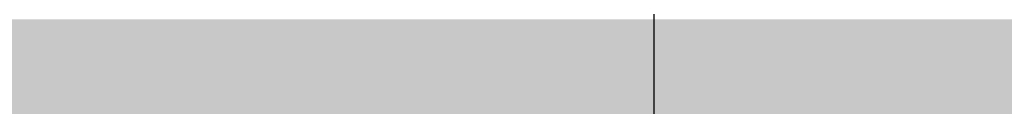
# Model space of a CAD drawing. Units: inches. Extents: x 2083 to 3317, y 1141 to 2115.
# Tile 47 of 256: x 2237.106 to 2238.294, y 1477.656 to 1477.759. Entities that reach past the tile are written whole.
import ezdxf

# ---------------------------------------------------------------- set-up
doc = ezdxf.new("R2010")
doc.units = ezdxf.units.IN
doc.layers.add('A-ANNO-DIMS', color=2, linetype='Continuous', lineweight=18)
doc.layers.add('A-WALL-PATT', color=251, linetype='Continuous', lineweight=13, true_color=0x636466)
doc.styles.get("Standard").update_dxf_attribs({"font": 'arial.ttf'})
doc.dimstyles.new('ISO-25', dxfattribs={"dimtxt": 12, "dimasz": 12, "dimexe": 1.25, "dimexo": 0.625, "dimtad": 1, "dimlunit": 3, "dimtxsty": 'Standard', "dimcen": 2.5, "dimadec": 0, "dimazin": 0, "dimtfac": 1, "dimtmove": 0, "dimatfit": 3, "dimfxl": 1, "dimarcsym": 0})

# ---------------------------------------------------------------- blocks, each defined once
blk = doc.blocks.new('*D30')
at = {"layer": 'A-ANNO-DIMS', "color": 0, "lineweight": -2, "transparency": 16777216}
for p, q in [((2240.0179, 1445.2738), (2240.0179, 1448.0455)), ((2254.3293, 1445.2738), (2254.3293, 1448.0455)), ((2228.0179, 1446.7955), (2216.0179, 1446.7955)), ((2240.0179, 1446.7955), (2254.3293, 1446.7955)), ((2266.3293, 1446.7955), (2413.7649, 1446.7955))]:
    blk.add_line(p, q, dxfattribs=at)
at = {"layer": 'A-ANNO-DIMS', "color": 0, "transparency": 16777216}
for points in [[(2228.0179, 1448.7955), (2228.0179, 1444.7955), (2240.0179, 1446.7955)], [(2266.3293, 1448.7955), (2266.3293, 1444.7955), (2254.3293, 1446.7955)]]:
    blk.add_solid(points, dxfattribs=at)
at = {"layer": 'Defpoints', "color": 0, "transparency": 16777216}
for p in [(2254.3293, 1446.7955), (2240.0179, 1444.6488), (2254.3293, 1444.6488)]:
    blk.add_point(p, dxfattribs=at)
at = {"layer": 'A-ANNO-DIMS', "color": 0, "transparency": 16777216, "insert": (2346.0471, 1453.6252), "char_height": 12, "attachment_point": 5}
blk.add_mtext('WC 1\'-2 1/2" TYP.', dxfattribs=at)
blk = doc.blocks.new('*D31')
at = {"layer": 'A-ANNO-DIMS', "color": 0, "lineweight": -2, "transparency": 16777216}
for p, q in [((2237.8711, 1456.6488), (2237.8711, 1541.9152)), ((2239.3929, 1444.6488), (2236.6211, 1444.6488)), ((2237.8711, 1431.5475), (2237.8711, 1444.6488)), ((2239.3929, 1431.5475), (2236.6211, 1431.5475)), ((2237.8711, 1419.5475), (2237.8711, 1407.5475))]:
    blk.add_line(p, q, dxfattribs=at)
at = {"layer": 'A-ANNO-DIMS', "color": 0, "transparency": 16777216}
for points in [[(2235.8711, 1456.6488), (2239.8711, 1456.6488), (2237.8711, 1444.6488)], [(2235.8711, 1419.5475), (2239.8711, 1419.5475), (2237.8711, 1431.5475)]]:
    blk.add_solid(points, dxfattribs=at)
at = {"layer": 'Defpoints', "color": 0, "transparency": 16777216}
for p in [(2237.8711, 1444.6488), (2240.0179, 1444.6488), (2240.0179, 1431.5475)]:
    blk.add_point(p, dxfattribs=at)
at = {"layer": 'A-ANNO-DIMS', "color": 0, "transparency": 16777216, "insert": (2231.2175, 1505.282), "char_height": 12, "attachment_point": 5, "rotation": 90}
blk.add_mtext('1\'-1" TYP.', dxfattribs=at)
blk = doc.blocks.new('*D62')
at = {"layer": 'A-ANNO-DIMS', "color": 0, "lineweight": -2, "transparency": 16777216}
for p, q in [((2235.9598, 1469.3864), (2235.9598, 1522.3614)), ((2379.9598, 1469.3864), (2379.9598, 1522.3614)), ((2247.9598, 1521.1114), (2367.9598, 1521.1114))]:
    blk.add_line(p, q, dxfattribs=at)
at = {"layer": 'A-ANNO-DIMS', "color": 0, "transparency": 16777216}
for points in [[(2247.9598, 1523.1114), (2247.9598, 1519.1114), (2235.9598, 1521.1114)], [(2367.9598, 1523.1114), (2367.9598, 1519.1114), (2379.9598, 1521.1114)]]:
    blk.add_solid(points, dxfattribs=at)
at = {"layer": 'Defpoints', "color": 0, "transparency": 16777216}
for p in [(2379.9598, 1521.1114), (2235.9598, 1468.7614), (2379.9598, 1468.7614)]:
    blk.add_point(p, dxfattribs=at)
at = {"layer": 'A-ANNO-DIMS', "color": 0, "transparency": 16777216, "insert": (2307.9598, 1527.8632), "char_height": 12, "attachment_point": 5}
blk.add_mtext('12\'-0"', dxfattribs=at)

msp = doc.modelspace()

# ---------------------------------------------------------------- hatches: boundary and pattern name
at = {"layer": 'A-WALL-PATT'}
h = msp.add_hatch(color=256, dxfattribs=at)
h.dxf.hatch_style = 1
h.paths.add_polyline_path([(3126.9598, 2020.7614), (2748.9598, 2020.7614), (2604.9598, 2020.7614), (2226.9598, 2020.7614), (2226.9598, 1702.7614), (2466.9598, 1702.7614), (2466.9598, 1582.7614), (2418.9598, 1582.7614), (2418.9598, 1477.7614), (2226.9598, 1477.7614), (2226.9598, 1263.2614), (2544.9598, 1263.2614), (2544.9598, 1411.7614), (2604.9598, 1411.7614), (2685.9598, 1411.7614), (2685.9598, 1420.7614), (2604.9598, 1420.7614), (2604.9598, 1573.7614), (2604.9598, 1702.7614), (2604.9598, 2011.7614), (2748.9598, 2011.7614), (2748.9598, 1702.7614), (2862.9598, 1702.7614), (2862.9598, 1621.7614), (2871.9598, 1621.7614), (2871.9598, 1702.7614), (2883.9598, 1702.7614), (2883.9598, 1706.9395, -0.026459), (2883.9598, 1711.7614), (2757.9598, 1711.7614), (2757.9598, 1807.7614), (2787.9598, 1807.7614), (2787.9598, 1812.2614), (2757.9598, 1812.2614), (2757.9598, 2011.7614), (2877.9598, 2011.7614), (2877.9598, 1812.2614), (2847.9598, 1812.2614), (2847.9598, 1807.7614), (2889.8357, 1807.7614), (2889.8357, 1812.2614), (2882.4598, 1812.2614), (2882.4598, 2011.7614), (3117.9598, 2011.7614), (3117.9598, 1812.2614), (2937.8357, 1812.2614), (2937.8357, 1807.7614), (2995.7098, 1807.7614), (2995.7098, 1796.1177), (3000.2098, 1796.1177), (3000.2098, 1807.7614), (3117.9598, 1807.7614), (3117.9598, 1711.7614), (3000.2098, 1711.7614), (3000.2098, 1760.1177), (2998.5727, 1760.1177, -0.020711), (2995.7098, 1760.1177), (2995.7098, 1711.7614), (2931.9598, 1711.7614), (2931.9598, 1702.7614), (3126.9598, 1702.7614)])
h.paths.add_polyline_path([(2471.4598, 2011.7614), (2471.4598, 1810.0114), (2462.7169, 1810.0114), (2462.7169, 1805.5114), (2505.9598, 1805.5114), (2505.9598, 1810.0114), (2475.9598, 1810.0114), (2475.9598, 2011.7614), (2595.9598, 2011.7614), (2595.9598, 1810.0114), (2565.9598, 1810.0114), (2565.9598, 1805.5114), (2595.9598, 1805.5114), (2595.9598, 1711.7614), (2235.9598, 1711.7614), (2235.9598, 1805.5114), (2353.7098, 1805.5114), (2353.7098, 1796.0542), (2358.2098, 1796.0542), (2358.2098, 1805.5114), (2414.7169, 1805.5114), (2414.7169, 1810.0114), (2235.9598, 1810.0114), (2235.9598, 2011.7614)], flags=16)
h.paths.add_polyline_path([(2270.2047, 1994.61), (2270.2047, 1970.61), (2246.2047, 1970.61), (2246.2047, 1994.61)], flags=0)
edge = h.paths.add_edge_path(flags=0)
edge.add_ellipse((2332.0274, 1899.7982), major_axis=(-3.043, 3.043), ratio=0.168252, start_angle=-161.3322, end_angle=-156.3071, ccw=False)
edge.add_ellipse((2333.082, 1898.7435), major_axis=(-1.0546, 1.0546), ratio=0.453532, start_angle=-123.371, end_angle=-94.1591)
edge = h.paths.add_edge_path(flags=0)
edge.add_ellipse((2332.0274, 1968.8763), major_axis=(3.043, 3.043), ratio=0.168252, start_angle=18.6678, end_angle=23.6929)
edge.add_spline(control_points=[(2332.9256, 1970.6911), (2332.2268, 1970.3361), (2330.8937, 1969.6589), (2328.4131, 1970.9321), (2327.2039, 1967.7487), (2324.7096, 1969.9556), (2322.5328, 1967.0124), (2320.0128, 1971.2958), (2317.6803, 1968.1578), (2316.0405, 1967.102), (2315.4269, 1966.8096)], knot_values=[0, 0, 0, 0, 2.267059, 4.324559, 6.685584, 8.878641, 11.121502, 14.300359, 17.755284, 19.732645, 19.732645, 19.732645, 19.732645], degree=3, periodic=0)
edge.add_ellipse((2332.0274, 1968.8763), major_axis=(3.043, 3.043), ratio=0.168252, start_angle=18.6678, end_angle=23.6929, ccw=False)
edge.add_ellipse((2333.082, 1969.9309), major_axis=(1.0546, 1.0546), ratio=0.453532, start_angle=56.629, end_angle=85.8409, ccw=False)
edge = h.paths.add_edge_path(flags=0)
edge.add_spline(control_points=[(2296.4283, 1967.9879), (2293.6278, 1965.3363), (2287.7036, 1959.7271), (2299.7439, 1949.9957), (2294.5326, 1935.6685), (2290.5732, 1920.6035), (2293.3941, 1909.9737), (2296.1854, 1904.9665)], knot_values=[0.099185, 0.099185, 0.099185, 0.099185, 0.345301, 0.619822, 0.982653, 1.386093, 1.810555, 1.810555, 1.810555, 1.810555], degree=3, periodic=0)
edge.add_spline(control_points=[(2296.1854, 1904.9665), (2297.3836, 1902.6193), (2298.001, 1901.9493), (2298.553, 1901.4682)], knot_values=[0.006246, 0.006246, 0.006246, 0.006246, 0.055476, 0.055476, 0.055476, 0.055476], degree=3, periodic=0)
edge.add_spline(control_points=[(2298.553, 1901.4682), (2297.2586, 1900.9232), (2295.2253, 1900.2321), (2293.0602, 1900.6142), (2292.1014, 1900.7884), (2292.0896, 1900.7906)], knot_values=[0.312835, 0.312835, 0.312835, 0.312835, 0.40178, 0.474987, 0.475903, 0.475903, 0.475903, 0.475903], degree=3, periodic=0)
edge.add_arc((2292.7936, 1904.6641), 3.937, 215.4209, 259.6982, ccw=False)
edge.add_spline(control_points=[(2289.5853, 1902.3823), (2289.4767, 1902.5351), (2289.3685, 1902.688), (2289.2609, 1902.8412)], knot_values=[0.102872, 0.102872, 0.102872, 0.102872, 0.116896, 0.116896, 0.116896, 0.116896], degree=3, periodic=0)
edge.add_spline(control_points=[(2289.2609, 1902.8412), (2288.6866, 1902.5502), (2287.64, 1902.0199), (2285.8813, 1901.874), (2283.853, 1901.5044), (2281.72, 1899.7105), (2278.467, 1899.4929), (2276.1571, 1901.8832), (2272.259, 1899.8041), (2267.7776, 1901.8432), (2262.2439, 1900.184), (2257.4149, 1901.7821), (2254.3184, 1900.7261), (2253.1783, 1900.3373)], knot_values=[0, 0, 0, 0, 1.907977, 3.477176, 5.261074, 7.972851, 11.680248, 13.717921, 16.939592, 22.789562, 27.502503, 33.595215, 37.145618, 37.145618, 37.145618, 37.145618], degree=3, periodic=0)
edge.add_line((2253.1783, 1900.3373), (2250.2442, 1902.8412))
edge.add_line((2250.2442, 1902.8412), (2250.2442, 1965.8333))
edge.add_line((2250.2442, 1965.8333), (2253.1783, 1968.3371))
edge.add_spline(control_points=[(2253.1783, 1968.3371), (2254.3184, 1967.9483), (2257.4149, 1966.8924), (2262.2439, 1968.4904), (2267.7776, 1966.8313), (2271.5267, 1968.5372), (2273.8759, 1967.8283), (2274.2067, 1967.7276)], knot_values=[0, 0, 0, 0, 0.09018, 0.244935, 0.364644, 0.513233, 0.537855, 0.537855, 0.537855, 0.537855], degree=3, periodic=0)
edge.add_arc((2274.3529, 1963.7933), 3.937, 72.0511, 92.1279, ccw=False)
edge.add_arc((2281.2969, 1985.23), 18.5963, 252.05113, 288.56572)
edge.add_arc((2292.3167, 1956.0289), 12.6461, 71.02679, 113.77822, ccw=False)
edge = h.paths.add_edge_path(flags=0)
edge.add_spline(control_points=[(2274.8994, 1951.8562), (2275.0662, 1951.6166), (2275.2327, 1951.3766), (2275.398, 1951.1359)], knot_values=[1.409916, 1.409916, 1.409916, 1.409916, 1.43159, 1.43159, 1.43159, 1.43159], degree=3, periodic=0)
edge.add_spline(control_points=[(2275.398, 1951.1359), (2275.7921, 1950.5619), (2276.1792, 1949.9838), (2276.5455, 1949.3971)], knot_values=[1.358238, 1.358238, 1.358238, 1.358238, 1.409916, 1.409916, 1.409916, 1.409916], degree=3, periodic=0)
edge.add_line((2276.5455, 1949.3971), (2277.4373, 1947.8622))
edge.add_spline(control_points=[(2277.4373, 1947.8622), (2276.3038, 1945.6731), (2274.6397, 1942.4269), (2274.6316, 1938.0939), (2272.7991, 1930.8515), (2274.3564, 1943.897), (2275.9477, 1947.9234), (2276.5455, 1949.3971)], knot_values=[0.005632, 0.005632, 0.005632, 0.005632, 0.186014, 0.266002, 0.357087, 0.59639, 0.739732, 0.739732, 0.739732, 0.739732], degree=3, periodic=0)
edge.add_spline(control_points=[(2276.5455, 1949.3971), (2276.1792, 1949.9838), (2275.7921, 1950.5619), (2275.398, 1951.1359)], knot_values=[1.358238, 1.358238, 1.358238, 1.358238, 1.409916, 1.409916, 1.409916, 1.409916], degree=3, periodic=0)
edge.add_spline(control_points=[(2275.398, 1951.1359), (2274.9425, 1950.0805), (2274.2078, 1948.0253), (2273.9346, 1944.8515), (2272.4685, 1937.6275), (2273.4662, 1945.6965), (2274.7006, 1951.0595), (2274.8994, 1951.8562)], knot_values=[0.104364, 0.104364, 0.104364, 0.104364, 0.189636, 0.269624, 0.36071, 0.600013, 0.644622, 0.644622, 0.644622, 0.644622], degree=3, periodic=0)
h.paths.add_polyline_path([(2269.1675, 1963.1276, -0.357527), (2268.1706, 1960.9764, -0.092561), (2268.1706, 1939.4363, -0.357527), (2269.1675, 1937.2851, -0.357527), (2267.0163, 1938.282, -0.164785), (2254.6856, 1938.282, -0.357527), (2252.5344, 1937.2851, -0.357527), (2253.5313, 1939.4363, -0.092561), (2253.5313, 1960.9764, -0.357527), (2252.5344, 1963.1276, -0.357527), (2254.6856, 1962.1307, -0.164785), (2267.0163, 1962.1307, -0.357527)], flags=0)
h.paths.add_polyline_path([(2248.8741, 1967.8018), (2248.8741, 1957.0277), (2249.4578, 1957.0277), (2249.4578, 1911.6468), (2248.8741, 1911.6468), (2248.8741, 1900.8727), (2246.5119, 1900.8727, 0.197327), (2244.1497, 1902.4569), (2244.1497, 1966.2176, 0.197327), (2246.5119, 1967.8018)], flags=0)
h.paths.add_polyline_path([(2269.1675, 1931.3893, -0.357527), (2268.1706, 1929.2381, -0.092561), (2268.1706, 1907.6981, -0.357527), (2269.1675, 1905.5469, -0.357527), (2267.0163, 1906.5438, -0.164785), (2254.6856, 1906.5438, -0.357527), (2252.5344, 1905.5469, -0.357527), (2253.5313, 1907.6981, -0.092561), (2253.5313, 1929.2381, -0.357527), (2252.5344, 1931.3893, -0.357527), (2254.6856, 1930.3925, -0.164785), (2267.0163, 1930.3925, -0.357527)], flags=0)
edge = h.paths.add_edge_path(flags=0)
edge.add_spline(control_points=[(2276.1969, 1906.7237), (2276.1681, 1909.0289), (2276.114, 1913.3719), (2270.5984, 1924.925), (2273.9052, 1919.0128), (2275.9217, 1916.2621), (2275.4746, 1912.4021), (2277.2579, 1910.3806), (2276.696, 1908.225), (2276.6462, 1906.813), (2276.6178, 1906.0084)], knot_values=[0, 0, 0, 0, 8.61026, 16.221274, 18.843057, 23.804898, 27.440828, 29.356102, 31.203478, 33.650687, 33.650687, 33.650687, 33.650687], degree=3, periodic=0)
edge.add_spline(control_points=[(2276.6178, 1906.0084), (2276.6233, 1905.6241), (2276.4977, 1904.6287), (2275.4418, 1903.8547), (2274.9373, 1903.0804), (2274.8591, 1902.8412)], knot_values=[0.156488, 0.156488, 0.156488, 0.156488, 0.184398, 0.231376, 0.250598, 0.250598, 0.250598, 0.250598], degree=3, periodic=0)
edge.add_line((2274.8591, 1902.8412), (2276.506, 1902.8412))
edge.add_spline(control_points=[(2276.506, 1902.8412), (2276.7883, 1903.0849), (2277.6651, 1904.1252), (2278.2495, 1904.3407), (2277.6539, 1908.5274), (2278.1557, 1906.2278), (2278.1005, 1905.2859), (2278.8467, 1904.069), (2277.8568, 1903.4149), (2277.8742, 1902.991), (2277.9036, 1902.8412)], knot_values=[0.059574, 0.059574, 0.059574, 0.059574, 0.080753, 0.103741, 0.16972, 0.176036, 0.207137, 0.240474, 0.262341, 0.27366, 0.27366, 0.27366, 0.27366], degree=3, periodic=0)
edge.add_line((2277.9036, 1902.8412), (2280.0298, 1902.8412))
edge.add_spline(control_points=[(2280.0298, 1902.8412), (2279.8882, 1903.0884), (2279.4993, 1903.9816), (2280.1523, 1905.9393), (2278.1036, 1909.6578), (2279.7624, 1907.1853), (2280.3279, 1904.8749), (2280.4851, 1903.4896), (2281.4633, 1903.2494), (2281.7583, 1902.9365), (2281.834, 1902.8412)], knot_values=[0.013856, 0.013856, 0.013856, 0.013856, 0.034874, 0.088867, 0.107879, 0.126738, 0.158714, 0.193757, 0.217487, 0.226722, 0.226722, 0.226722, 0.226722], degree=3, periodic=0)
edge.add_spline(control_points=[(2281.834, 1902.8412), (2281.7875, 1902.8267), (2281.647, 1902.783), (2281.3955, 1902.8595), (2281.0881, 1902.9852), (2280.7207, 1903.0609), (2280.3335, 1903.0257), (2280.1248, 1902.8989), (2280.0298, 1902.8412)], knot_values=[0, 0, 0, 0, 0.14413, 0.435517, 0.749276, 1.153046, 1.548371, 1.878348, 1.878348, 1.878348, 1.878348], degree=3, periodic=0)
edge.add_line((2280.0298, 1902.8412), (2277.9036, 1902.8412))
edge.add_spline(control_points=[(2277.9036, 1902.8412), (2277.8929, 1902.7959), (2277.8654, 1902.6796), (2277.6075, 1902.6875), (2277.2741, 1902.8007), (2276.8379, 1902.6198), (2276.5838, 1902.7893), (2276.506, 1902.8412)], knot_values=[0, 0, 0, 0, 0.127189, 0.326199, 0.628009, 1.24357, 1.515331, 1.515331, 1.515331, 1.515331], degree=3, periodic=0)
edge.add_line((2276.506, 1902.8412), (2274.8591, 1902.8412))
edge.add_spline(control_points=[(2274.8591, 1902.8412), (2274.8144, 1902.8986), (2274.7251, 1903.0134), (2274.4935, 1903.119), (2274.2443, 1902.9605), (2273.9371, 1903.1849), (2273.614, 1902.9831), (2273.4083, 1902.883), (2273.3223, 1902.8412)], knot_values=[0, 0, 0, 0, 0.21843, 0.436957, 0.687977, 0.990379, 1.398396, 1.69185, 1.69185, 1.69185, 1.69185], degree=3, periodic=0)
edge.add_spline(control_points=[(2273.3223, 1902.8412), (2273.6167, 1903.4457), (2274.274, 1904.5383), (2276.0272, 1904.5737), (2276.207, 1906.5836), (2276.1969, 1906.7237)], knot_values=[0.012227, 0.012227, 0.012227, 0.012227, 0.059472, 0.106218, 0.134458, 0.134458, 0.134458, 0.134458], degree=3, periodic=0)
h.paths.add_polyline_path([(2270.7761, 1897.7898), (2270.7761, 1873.7898), (2246.7761, 1873.7898), (2246.7761, 1897.7898)], flags=0)
h.paths.add_polyline_path([(2353.7098, 1760.0051), (2353.7098, 1760.0542), (2358.2098, 1760.0542, -0.033729)], flags=0)
h.paths.add_polyline_path([(2321.8191, 1737.5292), (2341.9953, 1737.5292, -0.414214), (2343.2033, 1736.3212), (2343.2033, 1721.0206, -0.414214), (2341.9953, 1719.8127), (2321.8191, 1719.8127, -0.414214), (2320.6112, 1721.0206), (2320.6112, 1736.3212, -0.414214)], flags=0)
h.paths.add_polyline_path([(2324.235, 1736.3212), (2339.5794, 1736.3212, -0.414214), (2341.9953, 1733.9053), (2341.9953, 1725.4497, -0.414214), (2339.5794, 1723.0338), (2333.6806, 1723.0338), (2333.8453, 1722.0455, -0.870646), (2335.4254, 1721.8259, -0.767327), (2333.9227, 1721.4232), (2331.291, 1721.4232, -0.767327), (2329.7883, 1721.8259, -0.870646), (2331.3684, 1722.0455), (2331.5331, 1723.0338), (2324.235, 1723.0338, -0.414214), (2321.8191, 1725.4497), (2321.8191, 1733.9053, -0.414214)], flags=0)
h.paths.add_polyline_path([(2570.4838, 1928.6154), (2589.6838, 1928.6154), (2590.1688, 1928.6154), (2590.1688, 1904.9934), (2570.4838, 1904.9934)], flags=0)
h.paths.add_polyline_path([(2574.4473, 1927.2638, -1), (2572.8288, 1927.2638, -1)], flags=0)
h.paths.add_polyline_path([(2573.0899, 1926.9409), (2573.925, 1927.776), (2574.1477, 1927.5533), (2573.3126, 1926.7182)], flags=0)
h.paths.add_polyline_path([(2578.7791, 1919.7296, -1), (2571.5917, 1919.7296, -1)], flags=0)
h.paths.add_polyline_path([(2578.3854, 1919.7296, -1), (2571.9854, 1919.7296, -1)], flags=0)
h.paths.add_polyline_path([(2331.5958, 1729.4762, -1), (2333.618, 1729.4762, -1)], flags=0)
h.paths.add_polyline_path([(2578.0342, 1927.2638, -1), (2576.4157, 1927.2638, -1)], flags=0)
h.paths.add_polyline_path([(2576.6889, 1927.5311), (2576.9116, 1927.7538), (2577.7467, 1926.9186), (2577.524, 1926.6959)], flags=0)
h.paths.add_polyline_path([(2578.1391, 1909.8595, -1), (2572.2317, 1909.8595, -1)], flags=0)
h.paths.add_polyline_path([(2577.7454, 1909.8595, -1), (2572.6254, 1909.8595, -1)], flags=0)
h.paths.add_polyline_path([(2583.7977, 1927.2638, -1), (2582.1792, 1927.2638, -1)], flags=0)
h.paths.add_polyline_path([(2582.7186, 1927.7538), (2583.5538, 1926.9186), (2583.3311, 1926.6959), (2582.4959, 1927.5311)], flags=0)
h.paths.add_polyline_path([(2582.4959, 1927.5311), (2582.7186, 1927.7538), (2583.5538, 1926.9186), (2583.3311, 1926.6959)], flags=0)
h.paths.add_polyline_path([(2587.7391, 1920.5296, -1), (2581.8317, 1920.5296, -1)], flags=0)
h.paths.add_polyline_path([(2587.3454, 1920.5296, -1), (2582.2254, 1920.5296, -1)], flags=0)
h.paths.add_polyline_path([(2587.3846, 1927.2638, -1), (2585.7661, 1927.2638, -1)], flags=0)
h.paths.add_polyline_path([(2586.082, 1926.9802), (2586.9172, 1927.8154), (2587.1399, 1927.5927), (2586.3047, 1926.7575)], flags=0)
h.paths.add_polyline_path([(2588.3791, 1910.6595, -1), (2581.1917, 1910.6595, -1)], flags=0)
h.paths.add_polyline_path([(2587.9854, 1910.6595, -1), (2581.5854, 1910.6595, -1)], flags=0)
h.paths.add_polyline_path([(2417.1677, 1729.4779), (2437.3439, 1729.4779, -0.414214), (2438.5519, 1728.2699), (2438.5519, 1712.9693, -0.414214), (2437.3439, 1711.7614), (2417.1677, 1711.7614, -0.414214), (2415.9598, 1712.9693), (2415.9598, 1728.2699, -0.414214)], flags=0)
h.paths.add_polyline_path([(2419.5836, 1728.2699), (2434.928, 1728.2699, -0.414214), (2437.3439, 1725.8541), (2437.3439, 1717.3984, -0.414214), (2434.928, 1714.9825), (2429.0292, 1714.9825), (2429.1939, 1713.9942, -0.870646), (2430.774, 1713.7746, -0.767327), (2429.2713, 1713.372), (2426.6396, 1713.372, -0.767327), (2425.1369, 1713.7746, -0.870646), (2426.717, 1713.9942), (2426.8817, 1714.9825), (2419.5836, 1714.9825, -0.414214), (2417.1677, 1717.3984), (2417.1677, 1725.8541, -0.414214)], flags=0)
h.paths.add_polyline_path([(2419.5836, 1728.2699), (2434.928, 1728.2699, -0.414214), (2437.3439, 1725.8541), (2437.3439, 1717.3984, -0.414214), (2434.928, 1714.9825), (2429.0292, 1714.9825), (2428.3581, 1719.009), (2427.5528, 1719.009), (2426.8817, 1714.9825), (2419.5836, 1714.9825, -0.414214), (2417.1677, 1717.3984), (2417.1677, 1725.8541, -0.414214)], flags=0)
h.paths.add_polyline_path([(2426.9444, 1721.4249, -1), (2428.9666, 1721.4249, -1)], flags=0)
h.paths.add_polyline_path([(2475.9598, 1702.7614), (2595.9598, 1702.7614), (2595.9598, 1582.7614), (2475.9598, 1582.7614)], flags=16)
h.paths.add_polyline_path([(2427.9598, 1573.7614), (2595.9598, 1573.7614), (2595.9598, 1468.7614), (2595.9598, 1420.7614), (2384.4598, 1420.7614), (2384.4598, 1468.7614), (2427.9598, 1468.7614)], flags=16)
h.paths.add_polyline_path([(2379.9598, 1468.7614), (2379.9598, 1420.7614), (2235.9598, 1420.7614), (2235.9598, 1468.7614)], flags=16)
h.paths.add_polyline_path([(2317.816, 1466.6958), (2337.9922, 1466.6958, -0.414214), (2339.2002, 1465.4878), (2339.2002, 1450.1872, -0.414214), (2337.9922, 1448.9792), (2317.816, 1448.9792, -0.414214), (2316.6081, 1450.1872), (2316.6081, 1465.4878, -0.414214)], flags=0)
h.paths.add_polyline_path([(2320.2319, 1465.4878), (2335.5763, 1465.4878, -0.414214), (2337.9922, 1463.0719), (2337.9922, 1454.6163, -0.414214), (2335.5763, 1452.2004), (2329.6775, 1452.2004), (2329.8422, 1451.212, -0.870646), (2331.4223, 1450.9925, -0.767327), (2329.9196, 1450.5898), (2327.2879, 1450.5898, -0.767327), (2325.7852, 1450.9925, -0.870646), (2327.3653, 1451.212), (2327.53, 1452.2004), (2320.2319, 1452.2004, -0.414214), (2317.816, 1454.6163), (2317.816, 1463.0719, -0.414214)], flags=0)
h.paths.add_polyline_path([(2320.2319, 1465.4878), (2335.5763, 1465.4878, -0.414214), (2337.9922, 1463.0719), (2337.9922, 1454.6163, -0.414214), (2335.5763, 1452.2004), (2329.6775, 1452.2004), (2329.0064, 1456.2269), (2328.2011, 1456.2269), (2327.53, 1452.2004), (2320.2319, 1452.2004, -0.414214), (2317.816, 1454.6163), (2317.816, 1463.0719, -0.414214)], flags=0)
h.paths.add_polyline_path([(2327.5926, 1458.6428, -1), (2329.6148, 1458.6428, -1)], flags=0)
h.paths.add_polyline_path([(2244.4117, 1433.3405), (2241.9209, 1433.3405, -0.414214), (2240.0179, 1435.2435), (2240.0179, 1440.9528, -0.414211), (2241.9209, 1442.8559), (2244.4117, 1442.8559, -1.976472)], flags=0)
h.paths.add_polyline_path([(2245.3569, 1434.3975, -0.414214), (2245.3569, 1441.7988, -2.144098)], flags=0)
h.paths.add_polyline_path([(2535.9598, 1416.2614), (2535.9598, 1272.2614), (2235.9598, 1272.2614), (2235.9598, 1416.2614)], flags=16)
h.paths.add_polyline_path([(2260.1196, 1384.2928), (2260.1196, 1362.0386), (2237.8654, 1362.0386), (2237.8654, 1384.2928)], flags=0)
edge = h.paths.add_edge_path(flags=0)
edge.add_line((2318.2518, 1362.0933), (2318.1458, 1362.001))
edge.add_ellipse((2317.4451, 1360.431), major_axis=(2.8216, 2.8216), ratio=0.168252, start_angle=18.6678, end_angle=20.9481, ccw=False)
edge.add_ellipse((2318.423, 1361.409), major_axis=(0.9779, 0.9779), ratio=0.453532, start_angle=56.629, end_angle=70.2262, ccw=False)
edge = h.paths.add_edge_path(flags=0)
edge.add_line((2319.1074, 1295.5711), (2319.015, 1295.6771))
edge.add_ellipse((2317.4451, 1296.3778), major_axis=(-2.8216, 2.8216), ratio=0.168252, start_angle=-161.3322, end_angle=-159.0519, ccw=False)
edge.add_ellipse((2318.423, 1295.3999), major_axis=(-0.9779, 0.9779), ratio=0.453532, start_angle=-123.371, end_angle=-109.7738)
edge = h.paths.add_edge_path(flags=0)
edge.add_spline(control_points=[(2284.2103, 1301.1702), (2284.5807, 1300.4447), (2284.8912, 1299.892), (2285.1596, 1299.461)], knot_values=[0.039066, 0.039066, 0.039066, 0.039066, 0.055476, 0.055476, 0.055476, 0.055476], degree=3, periodic=0)
edge.add_line((2285.1596, 1299.461), (2284.2103, 1301.1702))
edge = h.paths.add_edge_path(flags=0)
edge.add_line((2280.4125, 1297.298), (2283.37, 1297.0361))
edge.add_line((2283.37, 1297.0361), (2286.4057, 1297.9263))
edge.add_spline(control_points=[(2286.4057, 1297.9263), (2285.3055, 1297.4631), (2284.3448, 1297.1292), (2283.37, 1297.0361)], knot_values=[0.394369, 0.394369, 0.394369, 0.394369, 0.475903, 0.475903, 0.475903, 0.475903], degree=3, periodic=0)
edge.add_spline(control_points=[(2283.37, 1297.0361), (2283.2814, 1297.0277), (2282.3163, 1296.9573), (2281.3125, 1297.1345), (2280.4234, 1297.296), (2280.4125, 1297.298)], knot_values=[0.312835, 0.312835, 0.312835, 0.312835, 0.320246, 0.393453, 0.394369, 0.394369, 0.394369, 0.394369], degree=3, periodic=0)
edge = h.paths.add_edge_path(flags=0)
edge.add_line((2284.4356, 1359.6073), (2280.4463, 1355.328))
edge.add_line((2280.4463, 1355.328), (2279.58, 1351.0178))
edge.add_line((2279.58, 1351.0178), (2282.413, 1346.5804))
edge.add_spline(control_points=[(2282.413, 1346.5804), (2283.1533, 1345.5892), (2284.2529, 1344.0289), (2284.801, 1342.3872), (2284.9352, 1341.8055)], knot_values=[1.240098, 1.240098, 1.240098, 1.240098, 1.332892, 1.382712, 1.382712, 1.382712, 1.382712], degree=3, periodic=0)
edge.add_spline(control_points=[(2284.9352, 1341.8055), (2285.3191, 1340.1406), (2285.233, 1338.4092), (2284.9099, 1336.6541)], knot_values=[1.097484, 1.097484, 1.097484, 1.097484, 1.240098, 1.240098, 1.240098, 1.240098], degree=3, periodic=0)
edge.add_spline(control_points=[(2284.9099, 1336.6541), (2284.5868, 1334.899), (2284.0267, 1333.1203), (2283.4626, 1331.3606)], knot_values=[0.95487, 0.95487, 0.95487, 0.95487, 1.097484, 1.097484, 1.097484, 1.097484], degree=3, periodic=0)
edge.add_line((2283.4626, 1331.3606), (2281.8904, 1326.1534))
edge.add_line((2281.8904, 1326.1534), (2280.7563, 1321.0561))
edge.add_line((2280.7563, 1321.0561), (2280.2992, 1316.002))
edge.add_line((2280.2992, 1316.002), (2280.7159, 1310.9501))
edge.add_line((2280.7159, 1310.9501), (2282.0281, 1305.9721))
edge.add_line((2282.0281, 1305.9721), (2284.2103, 1301.1702))
edge.add_spline(control_points=[(2284.2103, 1301.1702), (2283.3407, 1302.7302), (2282.6119, 1304.3365), (2282.0281, 1305.9721)], knot_values=[0.099185, 0.099185, 0.099185, 0.099185, 0.241799, 0.241799, 0.241799, 0.241799], degree=3, periodic=0)
edge.add_spline(control_points=[(2282.0281, 1305.9721), (2281.4443, 1307.6078), (2281.0055, 1309.2728), (2280.7159, 1310.9501)], knot_values=[0.241799, 0.241799, 0.241799, 0.241799, 0.384413, 0.384413, 0.384413, 0.384413], degree=3, periodic=0)
edge.add_spline(control_points=[(2280.7159, 1310.9501), (2280.4332, 1312.5876), (2280.2894, 1314.277), (2280.2989, 1315.962), (2280.2992, 1316.002)], knot_values=[0.384413, 0.384413, 0.384413, 0.384413, 0.523647, 0.527028, 0.527028, 0.527028, 0.527028], degree=3, periodic=0)
edge.add_spline(control_points=[(2280.2992, 1316.002), (2280.3123, 1317.687), (2280.4779, 1319.3679), (2280.7563, 1321.0561)], knot_values=[0.527028, 0.527028, 0.527028, 0.527028, 0.669642, 0.669642, 0.669642, 0.669642], degree=3, periodic=0)
edge.add_spline(control_points=[(2280.7563, 1321.0561), (2281.0346, 1322.7443), (2281.4259, 1324.4396), (2281.8904, 1326.1534)], knot_values=[0.669642, 0.669642, 0.669642, 0.669642, 0.812256, 0.812256, 0.812256, 0.812256], degree=3, periodic=0)
edge.add_spline(control_points=[(2281.8904, 1326.1534), (2282.2644, 1327.5333), (2282.7879, 1329.2618), (2283.3528, 1331.0178), (2283.4626, 1331.3606)], knot_values=[0.812256, 0.812256, 0.812256, 0.812256, 0.927087, 0.95487, 0.95487, 0.95487, 0.95487], degree=3, periodic=0)
edge.add_line((2283.4626, 1331.3606), (2284.9099, 1336.6541))
edge.add_line((2284.9099, 1336.6541), (2284.9352, 1341.8055))
edge.add_line((2284.9352, 1341.8055), (2282.413, 1346.5804))
edge.add_spline(control_points=[(2282.413, 1346.5804), (2281.2751, 1348.1038), (2280.0784, 1349.5703), (2279.58, 1351.0178)], knot_values=[1.382712, 1.382712, 1.382712, 1.382712, 1.525326, 1.525326, 1.525326, 1.525326], degree=3, periodic=0)
edge.add_spline(control_points=[(2279.58, 1351.0178), (2279.4433, 1351.4147), (2279.1363, 1352.8569), (2279.7352, 1354.2904), (2280.4463, 1355.328)], knot_values=[1.525326, 1.525326, 1.525326, 1.525326, 1.564439, 1.667941, 1.667941, 1.667941, 1.667941], degree=3, periodic=0)
edge.add_spline(control_points=[(2280.4463, 1355.328), (2281.4261, 1356.7578), (2282.9308, 1358.1826), (2284.4356, 1359.6073)], knot_values=[1.667941, 1.667941, 1.667941, 1.667941, 1.810555, 1.810555, 1.810555, 1.810555], degree=3, periodic=0)
edge.add_arc((2280.6231, 1348.5182), 11.7262, 71.02679, 113.77822)
edge.add_arc((2270.4049, 1375.5952), 17.2436, 252.05113, 288.56572, ccw=False)
edge.add_arc((2263.966, 1355.7178), 3.6506, 72.0511, 92.1279)
edge.add_arc((2263.966, 1355.7178), 3.6506, 92.1279, 177.9851)
edge.add_spline(control_points=[(2260.3176, 1355.8462), (2260.2604, 1354.2207), (2260.5513, 1350.1865), (2262.9993, 1346.7663), (2264.4727, 1344.649)], knot_values=[1.43159, 1.43159, 1.43159, 1.43159, 1.564144, 1.770695, 1.770695, 1.770695, 1.770695], degree=3, periodic=0)
edge.add_line((2264.4727, 1344.649), (2264.9356, 1343.9825))
edge.add_spline(control_points=[(2263.801, 1340.2481), (2263.8432, 1340.5141), (2264.0672, 1341.7565), (2264.5127, 1343.0025), (2264.935, 1343.9811)], knot_values=[0.53657, 0.53657, 0.53657, 0.53657, 0.559349, 0.644622, 0.644622, 0.644622, 0.644622], degree=3, periodic=0)
edge.add_spline(control_points=[(2264.935, 1343.9811), (2265.1178, 1343.715), (2265.2989, 1343.4479), (2265.4768, 1343.1794)], knot_values=[1.384077, 1.384077, 1.384077, 1.384077, 1.409916, 1.409916, 1.409916, 1.409916], degree=3, periodic=0)
edge.add_spline(control_points=[(2265.4768, 1343.1794), (2265.6546, 1342.9108), (2265.8293, 1342.6408), (2265.9991, 1342.3688)], knot_values=[1.358238, 1.358238, 1.358238, 1.358238, 1.384077, 1.384077, 1.384077, 1.384077], degree=3, periodic=0)
edge.add_line((2265.9991, 1342.3688), (2266.826, 1340.9455))
edge.add_spline(control_points=[(2266.826, 1340.9455), (2268.8944, 1337.0897), (2271.3982, 1325.843), (2270.5162, 1310.5686), (2275.9194, 1301.8606), (2277.7895, 1299.1994)], knot_values=[0.116896, 0.116896, 0.116896, 0.116896, 0.472987, 1.050969, 1.313793, 1.313793, 1.313793, 1.313793], degree=3, periodic=0)
edge.add_spline(control_points=[(2277.7895, 1299.1994), (2277.8394, 1299.1285), (2277.8894, 1299.0575), (2277.9396, 1298.9866)], knot_values=[0.109884, 0.109884, 0.109884, 0.109884, 0.116896, 0.116896, 0.116896, 0.116896], degree=3, periodic=0)
edge.add_line((2277.9396, 1298.9866), (2277.7888, 1299.1991))
edge.add_spline(control_points=[(2277.7888, 1299.1991), (2277.2566, 1298.9294), (2276.2864, 1298.4379), (2275.0394, 1298.3344), (2274.3833, 1298.2389), (2274.2153, 1298.2093)], knot_values=[33.12187, 33.12187, 33.12187, 33.12187, 35.029056, 36.598255, 37.144827, 37.144827, 37.144827, 37.144827], degree=3, periodic=0)
edge.add_line((2274.2153, 1298.2093), (2273.0731, 1297.893))
edge.add_spline(control_points=[(2273.0731, 1297.893), (2272.3229, 1297.5798), (2271.0392, 1296.5105), (2269.2484, 1296.2261), (2268.4231, 1296.3747)], knot_values=[26.532584, 26.532584, 26.532584, 26.532584, 29.198919, 31.839101, 31.839101, 31.839101, 31.839101], degree=3, periodic=0)
edge.add_line((2268.4231, 1296.3747), (2263.8785, 1297.4575))
edge.add_spline(control_points=[(2263.8785, 1297.4575), (2263.5561, 1297.3594), (2261.8603, 1296.8387), (2260.2388, 1297.2824), (2258.9335, 1297.5165)], knot_values=[15.919551, 15.919551, 15.919551, 15.919551, 16.939592, 21.226067, 21.226067, 21.226067, 21.226067], degree=3, periodic=0)
edge.add_line((2258.9335, 1297.5165), (2254.0552, 1297.329))
edge.add_spline(control_points=[(2254.0552, 1297.329), (2253.7555, 1297.2958), (2252.1137, 1297.1652), (2250.4619, 1297.5442), (2249.1297, 1297.6679)], knot_values=[5.306517, 5.306517, 5.306517, 5.306517, 6.276435, 10.613034, 10.613034, 10.613034, 10.613034], degree=3, periodic=0)
edge.add_line((2249.1297, 1297.6679), (2244.3316, 1296.8778))
edge.add_line((2244.3316, 1296.8778), (2241.611, 1299.1994))
edge.add_line((2241.611, 1299.1994), (2241.611, 1357.6094))
edge.add_line((2241.611, 1357.6094), (2244.3316, 1359.9311))
edge.add_line((2244.3316, 1359.9311), (2252.7288, 1359.5427))
edge.add_spline(control_points=[(2252.7288, 1359.5427), (2252.8709, 1359.5464), (2253.3057, 1359.5482), (2253.7398, 1359.5143), (2254.0317, 1359.4824)], knot_values=[0.233291, 0.233291, 0.233291, 0.233291, 0.244935, 0.268927, 0.268927, 0.268927, 0.268927], degree=3, periodic=0)
edge.add_line((2254.0317, 1359.4824), (2259.5872, 1359.4164))
edge.add_spline(control_points=[(2259.5872, 1359.4164), (2260.6771, 1359.6285), (2262.0732, 1359.897), (2263.5237, 1359.4593), (2263.8304, 1359.366)], knot_values=[0.422516, 0.422516, 0.422516, 0.422516, 0.513233, 0.537855, 0.537855, 0.537855, 0.537855], degree=3, periodic=0)
edge.add_arc((2263.966, 1355.7178), 3.6506, 72.0511, 92.1279, ccw=False)
edge.add_arc((2270.4049, 1375.5952), 17.2436, 252.05113, 288.56572)
edge.add_arc((2280.6231, 1348.5182), 11.7262, 71.02679, 113.77822, ccw=False)
h.paths.add_polyline_path([(2240.3405, 1359.4347), (2240.3405, 1349.4444), (2240.8818, 1349.4444), (2240.8818, 1307.3645), (2240.3405, 1307.3645), (2240.3405, 1297.3741), (2238.1502, 1297.3741, 0.197327), (2235.9598, 1298.8431), (2235.9598, 1357.9657, 0.197327), (2238.1502, 1359.4347)], flags=0)
h.paths.add_polyline_path([(2259.1578, 1355.1005, -0.357527), (2258.2334, 1353.1058, -0.092561), (2258.2334, 1333.1326, -0.357527), (2259.1578, 1331.1379, -0.357527), (2257.1631, 1332.0622, -0.164785), (2245.7293, 1332.0622, -0.357527), (2243.7346, 1331.1379, -0.357527), (2244.6589, 1333.1326, -0.092561), (2244.6589, 1353.1058, -0.357527), (2243.7346, 1355.1005, -0.357527), (2245.7293, 1354.1761, -0.164785), (2257.1631, 1354.1761, -0.357527)], flags=0)
edge = h.paths.add_edge_path(flags=0)
edge.add_line((2265.9991, 1342.3688), (2266.826, 1340.9455))
edge.add_line((2266.826, 1340.9455), (2265.3076, 1337.8141))
edge.add_line((2265.3076, 1337.8141), (2264.3582, 1334.6529))
edge.add_line((2264.3582, 1334.6529), (2264.262, 1333.7997))
edge.add_spline(control_points=[(2264.262, 1333.7997), (2264.2084, 1333.1871), (2264.1621, 1332.3655), (2264.0071, 1331.4139), (2263.969, 1331.2018)], knot_values=[0.464444, 0.464444, 0.464444, 0.464444, 0.516691, 0.531608, 0.531608, 0.531608, 0.531608], degree=3, periodic=0)
edge.add_spline(control_points=[(2263.969, 1331.2018), (2263.7745, 1330.1189), (2263.4244, 1328.7908), (2263.2574, 1328.5307), (2263.234, 1328.5146)], knot_values=[0.372682, 0.372682, 0.372682, 0.372682, 0.44885, 0.464444, 0.464444, 0.464444, 0.464444], degree=3, periodic=0)
edge.add_spline(control_points=[(2263.234, 1328.5146), (2263.0964, 1328.4202), (2263.1312, 1329.3015), (2263.275, 1330.6157)], knot_values=[0.280919, 0.280919, 0.280919, 0.280919, 0.372682, 0.372682, 0.372682, 0.372682], degree=3, periodic=0)
edge.add_spline(control_points=[(2263.275, 1330.6157), (2263.4187, 1331.93), (2263.6715, 1333.6773), (2263.9699, 1335.315)], knot_values=[0.189157, 0.189157, 0.189157, 0.189157, 0.280919, 0.280919, 0.280919, 0.280919], degree=3, periodic=0)
edge.add_spline(control_points=[(2263.9699, 1335.315), (2264.1005, 1336.0322), (2264.4188, 1337.6219), (2264.7548, 1338.8644), (2264.9474, 1339.4911)], knot_values=[0.097394, 0.097394, 0.097394, 0.097394, 0.137578, 0.189157, 0.189157, 0.189157, 0.189157], degree=3, periodic=0)
edge.add_spline(control_points=[(2264.9474, 1339.4911), (2265.29, 1340.6061), (2265.6442, 1341.494), (2265.9991, 1342.3688)], knot_values=[0.005632, 0.005632, 0.005632, 0.005632, 0.097394, 0.097394, 0.097394, 0.097394], degree=3, periodic=0)
h.paths.add_polyline_path([(2259.1578, 1325.671, -0.357527), (2258.2334, 1323.6763, -0.092561), (2258.2334, 1303.7031, -0.357527), (2259.1578, 1301.7084, -0.357527), (2257.1631, 1302.6327, -0.164785), (2245.7293, 1302.6327, -0.357527), (2243.7346, 1301.7084, -0.357527), (2244.6589, 1303.7031, -0.092561), (2244.6589, 1323.6763, -0.357527), (2243.7346, 1325.671, -0.357527), (2245.7293, 1324.7466, -0.164785), (2257.1631, 1324.7466, -0.357527)], flags=0)
edge = h.paths.add_edge_path(flags=0)
edge.add_spline(control_points=[(2261.7089, 1317.3114), (2261.6795, 1317.4176), (2261.7619, 1317.3885), (2262.4907, 1316.0899), (2262.9622, 1315.3009)], knot_values=[14.955861, 14.955861, 14.955861, 14.955861, 16.221274, 18.694826, 18.694826, 18.694826, 18.694826], degree=3, periodic=0)
edge.add_spline(control_points=[(2262.9622, 1315.3009), (2262.9904, 1315.2536), (2263.7021, 1314.0674), (2264.349, 1313.1272), (2264.7301, 1312.1642)], knot_values=[18.694826, 18.694826, 18.694826, 18.694826, 18.843057, 22.433791, 22.433791, 22.433791, 22.433791], degree=3, periodic=0)
edge.add_spline(control_points=[(2264.7301, 1312.1642), (2264.8756, 1311.7964), (2265.1769, 1310.7698), (2265.1431, 1309.5593), (2265.2477, 1308.8242)], knot_values=[22.433791, 22.433791, 22.433791, 22.433791, 23.804898, 26.172756, 26.172756, 26.172756, 26.172756], degree=3, periodic=0)
edge.add_line((2265.2477, 1308.8242), (2265.8508, 1307.1719))
edge.add_spline(control_points=[(2265.8508, 1307.1719), (2266.065, 1306.8217), (2266.3844, 1306.3322), (2266.4244, 1305.7805), (2266.4204, 1305.6112)], knot_values=[28.062562, 28.062562, 28.062562, 28.062562, 29.356102, 29.911721, 29.911721, 29.911721, 29.911721], degree=3, periodic=0)
edge.add_spline(control_points=[(2266.4204, 1305.6112), (2266.4161, 1305.4326), (2266.394, 1305.25), (2266.3648, 1305.0659)], knot_values=[29.911721, 29.911721, 29.911721, 29.911721, 30.497837, 30.497837, 30.497837, 30.497837], degree=3, periodic=0)
edge.add_line((2266.3648, 1305.0659), (2266.0662, 1302.1363))
edge.add_spline(control_points=[(2266.0662, 1302.1363), (2266.0712, 1301.78), (2265.9981, 1301.2), (2265.6633, 1300.759), (2265.5089, 1300.5859)], knot_values=[0.156488, 0.156488, 0.156488, 0.156488, 0.184398, 0.203543, 0.203543, 0.203543, 0.203543], degree=3, periodic=0)
edge.add_line((2265.5089, 1300.5859), (2264.4353, 1299.1994))
edge.add_line((2264.4353, 1299.1994), (2265.9624, 1299.1994))
edge.add_line((2265.9624, 1299.1994), (2267.336, 1301.1753))
edge.add_line((2267.336, 1301.1753), (2267.3117, 1301.9862))
edge.add_spline(control_points=[(2267.3117, 1301.9862), (2267.2611, 1302.8624), (2267.1602, 1303.7371), (2267.2715, 1303.3259)], knot_values=[0.126229, 0.126229, 0.126229, 0.126229, 0.166617, 0.166617, 0.166617, 0.166617], degree=3, periodic=0)
edge.add_spline(control_points=[(2267.2715, 1303.3259), (2267.28, 1303.2943), (2267.3098, 1303.1754), (2267.3735, 1302.8836), (2267.4061, 1302.6828), (2267.4179, 1302.601)], knot_values=[0.166617, 0.166617, 0.166617, 0.166617, 0.16972, 0.176036, 0.180765, 0.180765, 0.180765, 0.180765], degree=3, periodic=0)
edge.add_spline(control_points=[(2267.7439, 1300.9875), (2267.6876, 1301.1509), (2267.4805, 1301.6567), (2267.4838, 1302.1448), (2267.4179, 1302.601)], knot_values=[0.180765, 0.180765, 0.180765, 0.180765, 0.193767, 0.220139, 0.220139, 0.220139, 0.220139], degree=3, periodic=0)
edge.add_line((2267.4179, 1302.601), (2267.7439, 1300.9875))
edge.add_spline(control_points=[(2267.7439, 1300.9875), (2267.832, 1300.7319), (2267.932, 1300.3099), (2267.5548, 1299.9745), (2267.4294, 1299.8292)], knot_values=[0.220139, 0.220139, 0.220139, 0.220139, 0.240474, 0.25489, 0.25489, 0.25489, 0.25489], degree=3, periodic=0)
edge.add_line((2267.4294, 1299.8292), (2267.2584, 1299.1994))
edge.add_line((2267.2584, 1299.1994), (2269.23, 1299.1994))
edge.add_spline(control_points=[(2269.23, 1299.1994), (2269.0987, 1299.4287), (2268.8428, 1300.0163), (2269.0116, 1300.9159), (2268.9468, 1301.6607)], knot_values=[0.013856, 0.013856, 0.013856, 0.013856, 0.034874, 0.067073, 0.067073, 0.067073, 0.067073], degree=3, periodic=0)
edge.add_line((2268.9468, 1301.6607), (2268.4316, 1303.6031))
edge.add_spline(control_points=[(2268.4316, 1303.6031), (2268.1756, 1304.1924), (2267.5962, 1305.2513), (2268.0407, 1304.6232), (2268.2514, 1304.2824)], knot_values=[0.090155, 0.090155, 0.090155, 0.090155, 0.107879, 0.120289, 0.120289, 0.120289, 0.120289], degree=3, periodic=0)
edge.add_spline(control_points=[(2268.2514, 1304.2824), (2268.3609, 1304.1053), (2269.0578, 1302.918), (2269.3827, 1301.5904), (2269.5214, 1300.7759), (2269.5752, 1300.5558)], knot_values=[0.120289, 0.120289, 0.120289, 0.120289, 0.126738, 0.158714, 0.173506, 0.173506, 0.173506, 0.173506], degree=3, periodic=0)
edge.add_line((2269.5752, 1300.5558), (2270.6858, 1299.4213))
edge.add_spline(control_points=[(2270.6858, 1299.4213), (2270.7672, 1299.3573), (2270.8379, 1299.2814), (2270.9029, 1299.1994)], knot_values=[0.21816, 0.21816, 0.21816, 0.21816, 0.226722, 0.226722, 0.226722, 0.226722], degree=3, periodic=0)
edge.add_line((2270.9372, 1299.1929), (2270.9029, 1299.1994))
edge.add_spline(control_points=[(2270.9029, 1299.1994), (2270.8598, 1299.186), (2270.7295, 1299.1455), (2270.4963, 1299.2164), (2270.2717, 1299.3083), (2270.121, 1299.348), (2270.0633, 1299.3596)], knot_values=[0.939174, 0.939174, 0.939174, 0.939174, 1.083304, 1.374691, 1.68845, 1.878348, 1.878348, 1.878348, 1.878348], degree=3, periodic=0)
edge.add_line((2270.0633, 1299.3596), (2269.23, 1299.1994))
edge.add_line((2269.23, 1299.1994), (2267.2584, 1299.1994))
edge.add_spline(control_points=[(2267.2584, 1299.1994), (2267.2484, 1299.1574), (2267.223, 1299.0497), (2266.9838, 1299.0569), (2266.8092, 1299.1162), (2266.6769, 1299.1091), (2266.6365, 1299.1048)], knot_values=[0.757665, 0.757665, 0.757665, 0.757665, 0.884854, 1.083864, 1.385675, 1.515331, 1.515331, 1.515331, 1.515331], degree=3, periodic=0)
edge.add_spline(control_points=[(2266.6365, 1299.1048), (2266.4852, 1299.0888), (2266.2358, 1299.0171), (2266.0346, 1299.1513), (2265.9624, 1299.1994)], knot_values=[0, 0, 0, 0, 0.485905, 0.757665, 0.757665, 0.757665, 0.757665], degree=3, periodic=0)
edge.add_line((2265.9624, 1299.1994), (2264.4353, 1299.1994))
edge.add_line((2264.4353, 1299.1994), (2263.8584, 1299.3671))
edge.add_spline(control_points=[(2263.8584, 1299.3671), (2263.8189, 1299.3709), (2263.7795, 1299.3857), (2263.7401, 1299.4015)], knot_values=[0.845925, 0.845925, 0.845925, 0.845925, 0.978627, 0.978627, 0.978627, 0.978627], degree=3, periodic=0)
edge.add_line((2263.7218, 1299.3964), (2263.0103, 1299.1994))
edge.add_spline(control_points=[(2263.0103, 1299.1994), (2263.2458, 1299.6829), (2263.506, 1300.1281), (2263.8735, 1300.408)], knot_values=[0.012227, 0.012227, 0.012227, 0.012227, 0.052971, 0.052971, 0.052971, 0.052971], degree=3, periodic=0)
edge.add_spline(control_points=[(2263.8735, 1300.408), (2263.9321, 1300.4527), (2264.0842, 1300.553), (2264.2552, 1300.6242), (2264.3597, 1300.6647)], knot_values=[0.052971, 0.052971, 0.052971, 0.052971, 0.059472, 0.069086, 0.069086, 0.069086, 0.069086], degree=3, periodic=0)
edge.add_line((2264.3597, 1300.6647), (2265.1419, 1301.0778))
edge.add_line((2265.1419, 1301.0778), (2265.6758, 1302.7996))
edge.add_line((2265.6758, 1302.7996), (2265.5407, 1305.7041))
edge.add_line((2265.5407, 1305.7041), (2264.8031, 1309.3277))
edge.add_line((2264.8031, 1309.3277), (2263.0405, 1314.0918))
edge.add_spline(control_points=[(2263.0405, 1314.0918), (2262.3836, 1315.6714), (2261.796, 1316.9977), (2261.7089, 1317.3114)], knot_values=[11.216896, 11.216896, 11.216896, 11.216896, 14.955861, 14.955861, 14.955861, 14.955861], degree=3, periodic=0)
h.paths.add_polyline_path([(2871.9598, 1416.2614), (2895.91, 1416.2614), (2895.91, 1420.7614), (2871.9598, 1420.7614), (2871.9598, 1501.7614), (2862.9598, 1501.7614), (2862.9598, 1420.7614), (2805.9598, 1420.7614), (2805.9598, 1411.7614), (2862.9598, 1411.7614), (2862.9598, 1263.2614), (3126.9598, 1263.2614), (3126.9598, 1411.7614), (3126.9598, 1486.7614), (2943.9598, 1486.7614), (2943.9598, 1477.7614), (2967.8603, 1477.7614), (2967.8603, 1420.7614), (2943.91, 1420.7614), (2943.91, 1416.2614), (3117.9598, 1416.2614), (3117.9598, 1420.7614), (2972.3603, 1420.7614), (2972.3603, 1477.7614), (3117.9598, 1477.7614), (3117.9598, 1420.7614), (3117.9598, 1272.2614), (2871.9598, 1272.2614)], flags=0)
h.paths.add_polyline_path([(2457.1256, 1485.9425), (2527.6027, 1485.9425), (2527.6027, 1537.6357), (2457.1256, 1537.6357)], flags=8)
h.paths.add_polyline_path([(2481.0051, 1609.9818), (2590.7658, 1609.9818), (2590.7658, 1682.0034), (2481.0051, 1682.0034)], flags=8)
h.paths.add_polyline_path([(2483.085, 1729.1268), (2553.562, 1729.1268), (2553.562, 1780.82), (2483.085, 1780.82)], flags=8)

# ---------------------------------------------------------------- dimensions: what is measured, and where the dimension line sits
at = {"layer": 'A-ANNO-DIMS'}
dim = msp.add_linear_dim(base=(2237.8711, 1444.6488), p1=(2240.0179, 1431.5475), p2=(2240.0179, 1444.6488), angle=90, text='<> TYP.', dimstyle='ISO-25', override={"dimdec": 1, "dimlfac": 1, "dimrnd": 0, "dimzin": 1, "dimdsep": 46, "dimlunit": 4, "dimfrac": 2}, dxfattribs=at)
dim.commit()
dim.dimension.update_dxf_attribs({"geometry": '*D31', "text_midpoint": (2231.2175, 1505.282)})
dim = msp.add_linear_dim(base=(2379.9598, 1521.1114), p1=(2235.9598, 1468.7614), p2=(2379.9598, 1468.7614), dimstyle='ISO-25', override={"dimdec": 1, "dimlfac": 1, "dimrnd": 0, "dimzin": 1, "dimdsep": 46, "dimlunit": 4, "dimfrac": 2}, dxfattribs=at)
dim.commit()
dim.dimension.update_dxf_attribs({"geometry": '*D62', "text_midpoint": (2307.9598, 1527.8632)})
dim = msp.add_linear_dim(base=(2254.3293, 1446.7955), p1=(2240.0179, 1444.6488), p2=(2254.3293, 1444.6488), text='WC <> TYP.', dimstyle='ISO-25', override={"dimdec": 1, "dimlfac": 1, "dimrnd": 0, "dimzin": 1, "dimdsep": 46, "dimlunit": 4, "dimfrac": 2}, dxfattribs=at)
dim.commit()
dim.dimension.update_dxf_attribs({"geometry": '*D30', "text_midpoint": (2346.0471, 1453.6252)})

doc.saveas('drawing.dxf')
